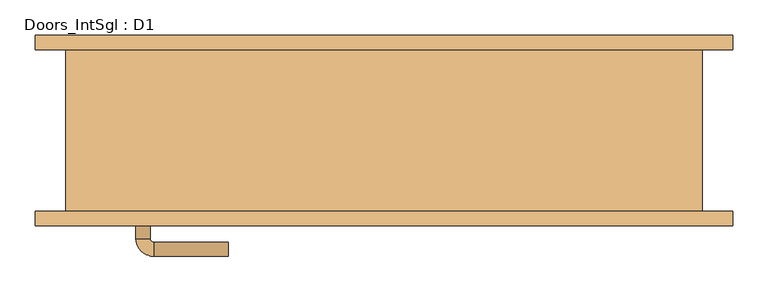
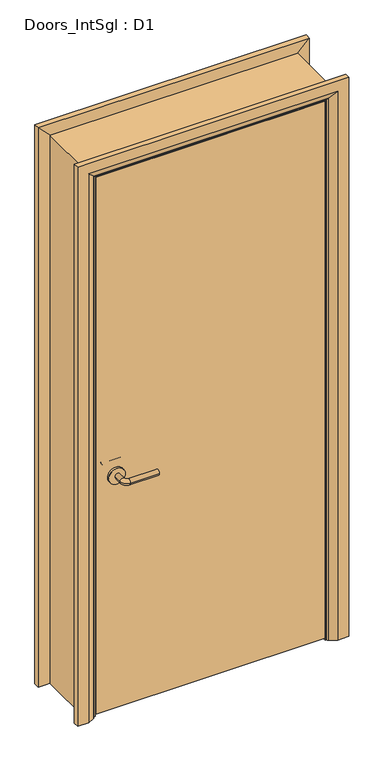
"""IFC4 building model written with IfcOpenShell, lengths in millimetres: door geometry, Doors_IntSgl : D1."""

from ifc_helpers import new_model, si_unit, point, frame, frame_2d, origin, place, context, project, spatial, polyline, circle_curve, ellipse_curve, trimmed, segment, composite_curve, outline, extrude, faceted_brep, source, transform, mapped, element, save
from ifc_brep_helpers import plane_surface, cylinder_surface, revolved_surface, advanced_brep


def doors_intsgl_d1_5aeab8eb(model_context):
    return source(origin(), model_context, "Body", "SolidModel", [
        advanced_brep(
        [(-350.2, -68.3, 900.0), (-330.2, -68.3, 900.0), (-350.2, -38.3, 900.0), (-330.2, -38.3, 900.0), (-325.2, -33.3, 900.0), (-325.2, -13.3, 900.0), (-220.2, -13.3, 900.0), (-220.2, -33.3, 900.0)],
        [
            (0, 1, circle_curve(frame((-340.2, -68.3, 900.0), z_axis=(0.0, -1.0, 0.0), x_axis=(1.0, 0.0, 0.0)), 10.0)),
            (1, 0, circle_curve(frame((-340.2, -68.3, 900.0), z_axis=(0.0, -1.0, 0.0), x_axis=(1.0, 0.0, 0.0)), 10.0)),
            (0, 2),
            (2, 3, circle_curve(frame((-340.2, -38.3, 900.0), z_axis=(0.0, -1.0, 0.0), x_axis=(1.0, 0.0, 0.0)), 10.0)),
            (3, 1),
            (3, 2, circle_curve(frame((-340.2, -38.3, 900.0), z_axis=(0.0, -1.0, 0.0), x_axis=(1.0, 0.0, 0.0)), 10.0)),
            (4, 3, circle_curve(frame((-325.2, -38.3, 900.0), z_axis=(0.0, 0.0, 1.0), x_axis=(-1.0, 0.0, 0.0)), 5.0)),
            (2, 5, circle_curve(frame((-325.2, -38.3, 900.0), z_axis=(0.0, 0.0, -1.0), x_axis=(-1.0, 0.0, 0.0)), 25.0)),
            (5, 4, circle_curve(frame((-325.2, -23.3, 900.0), z_axis=(-1.0, 0.0, 0.0), x_axis=(0.0, -1.0, 0.0)), 10.0)),
            (4, 5, circle_curve(frame((-325.2, -23.3, 900.0), z_axis=(-1.0, 0.0, 0.0), x_axis=(0.0, -1.0, 0.0)), 10.0)),
            (6, 7, circle_curve(frame((-220.2, -23.3, 900.0), z_axis=(1.0, 0.0, 0.0), x_axis=(0.0, -1.0, 0.0)), 10.0)),
            (7, 6, circle_curve(frame((-220.2, -23.3, 900.0), z_axis=(1.0, 0.0, 0.0), x_axis=(0.0, -1.0, 0.0)), 10.0)),
            (5, 6),
            (7, 4),
        ],
        [
            plane_surface(frame((-340.2, -68.3, 900.0), z_axis=(0.0, -1.0, 0.0), x_axis=(0.0, 0.0, 1.0))),
            cylinder_surface(frame((-340.2, -68.3, 900.0), z_axis=(0.0, -1.0, 0.0), x_axis=(1.0, 0.0, 0.0)), 10.0),
            revolved_surface(trimmed(ellipse_curve(frame((-340.2, -38.3, 900.0), z_axis=(0.0, -1.0, 0.0), x_axis=(1.0, 0.0, 0.0)), 10.0, 10.0), [point((-350.2, -38.3, 900.0))], [point((-330.2, -38.3, 900.0))], True, "CARTESIAN"), (-325.2, -38.3, 900.0), (0.0, 0.0, -1.0)),
            revolved_surface(trimmed(ellipse_curve(frame((-340.2, -38.3, 900.0), z_axis=(0.0, -1.0, 0.0), x_axis=(1.0, 0.0, 0.0)), 10.0, 10.0), [point((-330.2, -38.3, 900.0))], [point((-350.2, -38.3, 900.0))], True, "CARTESIAN"), (-325.2, -38.3, 900.0), (0.0, 0.0, -1.0)),
            plane_surface(frame((-220.2, -23.3, 900.0), z_axis=(1.0, 0.0, 0.0), x_axis=(0.0, 0.0, 1.0))),
            cylinder_surface(frame((-325.2, -23.3, 900.0), z_axis=(-1.0, 0.0, 0.0), x_axis=(0.0, -1.0, 0.0)), 10.0),
        ],
        [
            (0, [[1, 2]]),
            (1, [[-1, 3, 4, 5]]),
            (1, [[-2, -5, 6, -3]]),
            (2, [[7, -4, 8, 9]]),
            (3, [[-8, -6, -7, 10]]),
            (4, [[11, 12]]),
            (5, [[-9, 13, -12, 14]]),
            (5, [[-10, -14, -11, -13]]),
        ],
    ),
        extrude(outline(composite_curve([segment(trimmed(circle_curve(frame_2d((900.0, -342.7)), 30.0), [point((900.0, -372.7))], [point((900.0, -312.7))], False, "CARTESIAN"), True, "CONTINUOUS"), segment(trimmed(circle_curve(frame_2d((900.0, -342.7)), 30.0), [point((900.0, -312.7))], [point((900.0, -372.7))], False, "CARTESIAN"), True, "CONTINUOUS")], self_intersect=False)), frame((0.0, -76.3, 0.0), z_axis=(0.0, 1.0, 0.0), x_axis=(0.0, 0.0, 1.0)), (0.0, 0.0, 1.0), 8.0),
        advanced_brep(
        [(-350.2, -122.3, 900.0), (-330.2, -122.3, 900.0), (-330.2, -152.3, 900.0), (-350.2, -152.3, 900.0), (-325.2, -157.3, 900.0), (-325.2, -177.3, 900.0), (-220.2, -177.3, 900.0), (-220.2, -157.3, 900.0)],
        [
            (0, 1, circle_curve(frame((-340.2, -122.3, 900.0), z_axis=(0.0, 1.0, 0.0), x_axis=(1.0, 0.0, 0.0)), 10.0)),
            (1, 0, circle_curve(frame((-340.2, -122.3, 900.0), z_axis=(0.0, 1.0, 0.0), x_axis=(1.0, 0.0, 0.0)), 10.0)),
            (1, 2),
            (2, 3, circle_curve(frame((-340.2, -152.3, 900.0), z_axis=(0.0, 1.0, 0.0), x_axis=(1.0, 0.0, 0.0)), 10.0)),
            (3, 0),
            (3, 2, circle_curve(frame((-340.2, -152.3, 900.0), z_axis=(0.0, 1.0, 0.0), x_axis=(1.0, 0.0, 0.0)), 10.0)),
            (4, 5, circle_curve(frame((-325.2, -167.3, 900.0), z_axis=(-1.0, 0.0, 0.0), x_axis=(0.0, 1.0, 0.0)), 10.0)),
            (5, 3, circle_curve(frame((-325.2, -152.3, 900.0), z_axis=(0.0, 0.0, -1.0), x_axis=(-1.0, 0.0, 0.0)), 25.0)),
            (2, 4, circle_curve(frame((-325.2, -152.3, 900.0), z_axis=(0.0, 0.0, 1.0), x_axis=(-1.0, 0.0, 0.0)), 5.0)),
            (5, 4, circle_curve(frame((-325.2, -167.3, 900.0), z_axis=(-1.0, 0.0, 0.0), x_axis=(0.0, 1.0, 0.0)), 10.0)),
            (6, 7, circle_curve(frame((-220.2, -167.3, 900.0), z_axis=(1.0, 0.0, 0.0), x_axis=(0.0, 1.0, 0.0)), 10.0)),
            (7, 6, circle_curve(frame((-220.2, -167.3, 900.0), z_axis=(1.0, 0.0, 0.0), x_axis=(0.0, 1.0, 0.0)), 10.0)),
            (4, 7),
            (6, 5),
        ],
        [
            plane_surface(frame((-340.2, -122.3, 900.0), z_axis=(0.0, 1.0, 0.0), x_axis=(0.0, 0.0, 1.0))),
            cylinder_surface(frame((-340.2, -122.3, 900.0), z_axis=(0.0, 1.0, 0.0), x_axis=(1.0, 0.0, 0.0)), 10.0),
            revolved_surface(trimmed(ellipse_curve(frame((-340.2, -152.3, 900.0), z_axis=(0.0, -1.0, 0.0), x_axis=(1.0, 0.0, 0.0)), 10.0, 10.0), [point((-350.2, -152.3, 900.0))], [point((-330.2, -152.3, 900.0))], True, "CARTESIAN"), (-325.2, -152.3, 900.0), (0.0, 0.0, -1.0)),
            revolved_surface(trimmed(ellipse_curve(frame((-340.2, -152.3, 900.0), z_axis=(0.0, -1.0, 0.0), x_axis=(1.0, 0.0, 0.0)), 10.0, 10.0), [point((-330.2, -152.3, 900.0))], [point((-350.2, -152.3, 900.0))], True, "CARTESIAN"), (-325.2, -152.3, 900.0), (0.0, 0.0, -1.0)),
            plane_surface(frame((-220.2, -167.3, 900.0), z_axis=(1.0, 0.0, 0.0), x_axis=(0.0, 0.0, 1.0))),
            cylinder_surface(frame((-325.2, -167.3, 900.0), z_axis=(-1.0, 0.0, 0.0), x_axis=(0.0, 1.0, 0.0)), 10.0),
        ],
        [
            (0, [[1, 2]]),
            (1, [[3, 4, 5, -2]]),
            (1, [[-5, 6, -3, -1]]),
            (2, [[7, 8, -4, 9]]),
            (3, [[10, -9, -6, -8]]),
            (4, [[11, 12]]),
            (5, [[13, -11, 14, -7]]),
            (5, [[-14, -12, -13, -10]]),
        ],
    ),
        extrude(outline(composite_curve([segment(trimmed(circle_curve(frame_2d((900.0, -342.7)), 30.0), [point((900.0, -372.7))], [point((900.0, -312.7))], False, "CARTESIAN"), True, "CONTINUOUS"), segment(trimmed(circle_curve(frame_2d((900.0, -342.7)), 30.0), [point((900.0, -312.7))], [point((900.0, -372.7))], False, "CARTESIAN"), True, "CONTINUOUS")], self_intersect=False)), frame((0.0, -122.3, 0.0), z_axis=(0.0, 1.0, 0.0), x_axis=(0.0, 0.0, 1.0)), (0.0, 0.0, 1.0), 8.0),
        extrude(outline(polyline([(415.2, -76.3), (415.2, -114.3), (-415.2, -114.3), (-415.2, -76.3), (415.2, -76.3)])), frame((0.0, 0.0, 8.0), z_axis=(0.0, 0.0, 1.0), x_axis=(1.0, 0.0, 0.0)), (0.0, 0.0, 1.0), 2060.0),
        advanced_brep(
        [(492.2, -134.3, 0.0), (452.2, -134.3, 0.0), (426.2, -120.3, 0.0), (422.2, -114.3, 0.0), (492.2, -114.3, 0.0), (492.2, -114.3, 2145.0), (492.2, -134.3, 2145.0), (422.2, -114.3, 2075.0), (-422.2, -114.3, 2075.0), (-422.2, -114.3, 0.0), (-492.2, -114.3, 0.0), (-492.2, -114.3, 2145.0), (426.2, -120.3, 2079.0), (452.2, -134.3, 2105.0), (-492.2, -134.3, 2145.0), (-492.2, -134.3, 0.0), (-452.2, -134.3, 0.0), (-452.2, -134.3, 2105.0), (-426.2, -120.3, 0.0), (-426.2, -120.3, 2079.0)],
        [
            (0, 1),
            (1, 2),
            (2, 3, circle_curve(frame((430.2, -113.3, 0.0), z_axis=(0.0, 0.0, -1.0), x_axis=(1.0, 0.0, 0.0)), 8.0622577)),
            (3, 4),
            (4, 0),
            (4, 5),
            (5, 6),
            (6, 0),
            (3, 7),
            (7, 8),
            (8, 9),
            (9, 10),
            (10, 11),
            (11, 5),
            (2, 12),
            (12, 7, ellipse_curve(frame((430.2, -113.3, 2083.0), z_axis=(0.7071067811865475, 0.0, -0.7071067811865475), x_axis=(-0.7071067811865474, 0.0, -0.7071067811865476)), 11.4017543, 8.0622577)),
            (1, 13),
            (13, 12),
            (6, 14),
            (14, 15),
            (15, 16),
            (16, 17),
            (17, 13),
            (10, 15),
            (14, 11),
            (9, 18, circle_curve(frame((-430.2, -113.3, 0.0), z_axis=(0.0, 0.0, -1.0), x_axis=(-1.0, 0.0, 0.0)), 8.0622577)),
            (18, 16),
            (19, 18),
            (8, 19, ellipse_curve(frame((-430.2, -113.3, 2083.0), z_axis=(-0.7071067811865475, 0.0, -0.7071067811865475), x_axis=(-0.7071067811865474, 0.0, 0.7071067811865476)), 11.4017543, 8.0622577)),
            (19, 17),
            (12, 19),
        ],
        [
            plane_surface(frame((422.2, -114.3, 0.0), z_axis=(0.0, 0.0, -1.0), x_axis=(0.0, 1.0, 0.0))),
            plane_surface(frame((492.2, -134.3, 0.0), z_axis=(1.0, 0.0, 0.0), x_axis=(0.0, 0.0, 1.0))),
            plane_surface(frame((492.2, -114.3, 0.0), z_axis=(0.0, 1.0, 0.0), x_axis=(0.0, 0.0, 1.0))),
            cylinder_surface(frame((430.2, -113.3, 0.0), z_axis=(0.0, 0.0, -1.0), x_axis=(1.0, 0.0, 0.0)), 8.0622577),
            plane_surface(frame((426.2, -120.3, 0.0), z_axis=(-0.4740998230350126, -0.880471099922178, 0.0), x_axis=(0.0, 0.0, 1.0))),
            plane_surface(frame((452.2, -134.3, 0.0), z_axis=(0.0, -1.0, 0.0), x_axis=(0.0, 0.0, 1.0))),
            plane_surface(frame((-492.2, -134.3, 2145.0), z_axis=(-1.0, 0.0, 0.0), x_axis=(0.0, 0.0, -1.0))),
            plane_surface(frame((-422.2, -114.3, 0.0), z_axis=(0.0, 0.0, -1.0), x_axis=(0.0, 1.0, 0.0))),
            cylinder_surface(frame((-430.2, -113.3, 2075.0), z_axis=(0.0, 0.0, 1.0), x_axis=(-1.0, 0.0, 0.0)), 8.0622577),
            plane_surface(frame((-426.2, -120.3, 2079.0), z_axis=(0.47409982303501824, -0.8804710999221749, 0.0), x_axis=(0.0, 0.0, -1.0))),
            plane_surface(frame((492.2, -134.3, 2145.0), z_axis=(0.0, 0.0, 1.0), x_axis=(-1.0, 0.0, 0.0))),
            cylinder_surface(frame((422.2, -113.3, 2083.0), z_axis=(1.0, 0.0, 0.0), x_axis=(0.0, 0.0, 1.0)), 8.0622577),
            plane_surface(frame((426.2, -120.3, 2079.0), z_axis=(0.0, -0.8804710999221764, -0.4740998230350154), x_axis=(-1.0, 0.0, 0.0))),
        ],
        [
            (0, [[1, 2, 3, 4, 5]]),
            (1, [[6, 7, 8, -5]]),
            (2, [[9, 10, 11, 12, 13, 14, -6, -4]]),
            (3, [[15, 16, -9, -3]]),
            (4, [[17, 18, -15, -2]]),
            (5, [[-8, 19, 20, 21, 22, 23, -17, -1]]),
            (6, [[-13, 24, -20, 25]]),
            (7, [[-24, -12, 26, 27, -21]]),
            (8, [[28, -26, -11, 29]]),
            (9, [[-22, -27, -28, 30]]),
            (10, [[-14, -25, -19, -7]]),
            (11, [[31, -29, -10, -16]]),
            (12, [[-23, -30, -31, -18]]),
        ],
    ),
        extrude(outline(polyline([(0.0, -398.2), (2051.0, -398.2), (2051.0, 398.2), (0.0, 398.2), (0.0, 417.2), (2070.0, 417.2), (2070.0, -417.2), (0.0, -417.2), (0.0, -398.2)])), frame((0.0, -74.3, 0.0), z_axis=(0.0, 1.0, 0.0), x_axis=(0.0, 0.0, 1.0)), (0.0, 0.0, 1.0), 32.0),
        advanced_brep(
        [(-492.2, 134.3, 0.0), (-452.2, 134.3, 0.0), (-426.2, 120.3, 0.0), (-422.2, 114.3, 0.0), (-492.2, 114.3, 0.0), (-492.2, 114.3, 2145.0), (-492.2, 134.3, 2145.0), (-422.2, 114.3, 2075.0), (-426.2, 120.3, 2079.0), (-452.2, 134.3, 2105.0), (492.2, 134.3, 0.0), (492.2, 114.3, 0.0), (422.2, 114.3, 0.0), (426.2, 120.3, 0.0), (452.2, 134.3, 0.0), (492.2, 134.3, 2145.0), (452.2, 134.3, 2105.0), (426.2, 120.3, 2079.0), (422.2, 114.3, 2075.0), (492.2, 114.3, 2145.0)],
        [
            (0, 1),
            (1, 2),
            (2, 3, circle_curve(frame((-430.2, 113.3, 0.0), z_axis=(0.0, 0.0, -1.0), x_axis=(-1.0, 0.0, 0.0)), 8.0622577)),
            (3, 4),
            (4, 0),
            (4, 5),
            (5, 6),
            (6, 0),
            (3, 7),
            (7, 5),
            (2, 8),
            (8, 7, ellipse_curve(frame((-430.2, 113.3, 2083.0), z_axis=(-0.7071067811865475, 0.0, -0.7071067811865475), x_axis=(0.7071067811865474, 0.0, -0.7071067811865476)), 11.4017543, 8.0622577)),
            (1, 9),
            (9, 8),
            (6, 9),
            (10, 11),
            (11, 12),
            (12, 13, circle_curve(frame((430.2, 113.3, 0.0), z_axis=(0.0, 0.0, -1.0), x_axis=(1.0, 0.0, 0.0)), 8.0622577)),
            (13, 14),
            (14, 10),
            (15, 10),
            (14, 16),
            (16, 15),
            (13, 17),
            (17, 16),
            (12, 18),
            (18, 17, ellipse_curve(frame((430.2, 113.3, 2083.0), z_axis=(0.7071067811865475, 0.0, -0.7071067811865475), x_axis=(0.7071067811865474, 0.0, 0.7071067811865476)), 11.4017543, 8.0622577)),
            (11, 19),
            (19, 18),
            (15, 19),
            (5, 19),
            (15, 6),
            (7, 18),
            (8, 17),
            (9, 16),
        ],
        [
            plane_surface(frame((-422.2, 187.1010989, 0.0), z_axis=(0.0, 0.0, -1.0), x_axis=(1.0, 0.0, 0.0))),
            plane_surface(frame((-492.2, 134.3, 0.0), z_axis=(-1.0, 0.0, 0.0), x_axis=(0.0, 0.0, 1.0))),
            plane_surface(frame((-492.2, 114.3, 0.0), z_axis=(0.0, -1.0, 0.0), x_axis=(0.0, 0.0, 1.0))),
            cylinder_surface(frame((-430.2, 113.3, 0.0), z_axis=(0.0, 0.0, -1.0), x_axis=(-1.0, 0.0, 0.0)), 8.0622577),
            plane_surface(frame((-426.2, 120.3, 0.0), z_axis=(0.4740998230350183, 0.8804710999221749, 0.0), x_axis=(0.0, 0.0, 1.0))),
            plane_surface(frame((-452.2, 134.3, 0.0), z_axis=(0.0, 1.0, 0.0), x_axis=(0.0, 0.0, 1.0))),
            plane_surface(frame((422.2, 187.1010989, 0.0), z_axis=(0.0, 0.0, -1.0), x_axis=(-1.0, 0.0, 0.0))),
            plane_surface(frame((452.2, 134.3, 2105.0), z_axis=(0.0, 1.0, 0.0), x_axis=(0.0, 0.0, -1.0))),
            plane_surface(frame((426.2, 120.3, 2079.0), z_axis=(-0.4740998230350183, 0.8804710999221749, 0.0), x_axis=(0.0, 0.0, -1.0))),
            cylinder_surface(frame((430.2, 113.3, 2075.0), z_axis=(0.0, 0.0, 1.0), x_axis=(1.0, 0.0, 0.0)), 8.0622577),
            plane_surface(frame((492.2, 114.3, 2145.0), z_axis=(0.0, -1.0, 0.0), x_axis=(0.0, 0.0, -1.0))),
            plane_surface(frame((492.2, 134.3, 2145.0), z_axis=(1.0, 0.0, 0.0), x_axis=(0.0, 0.0, -1.0))),
            plane_surface(frame((-492.2, 134.3, 2145.0), z_axis=(0.0, 0.0, 1.0), x_axis=(1.0, 0.0, 0.0))),
            plane_surface(frame((-492.2, 114.3, 2145.0), z_axis=(0.0, -1.0, 0.0), x_axis=(1.0, 0.0, 0.0))),
            cylinder_surface(frame((-422.2, 113.3, 2083.0), z_axis=(-1.0, 0.0, 0.0), x_axis=(0.0, 0.0, 1.0)), 8.0622577),
            plane_surface(frame((-426.2, 120.3, 2079.0), z_axis=(0.0, 0.8804710999221749, -0.4740998230350183), x_axis=(1.0, 0.0, 0.0))),
            plane_surface(frame((-452.2, 134.3, 2105.0), z_axis=(0.0, 1.0, 0.0), x_axis=(1.0, 0.0, 0.0))),
        ],
        [
            (0, [[1, 2, 3, 4, 5]]),
            (1, [[6, 7, 8, -5]]),
            (2, [[9, 10, -6, -4]]),
            (3, [[11, 12, -9, -3]]),
            (4, [[13, 14, -11, -2]]),
            (5, [[-8, 15, -13, -1]]),
            (6, [[16, 17, 18, 19, 20]]),
            (7, [[21, -20, 22, 23]]),
            (8, [[-22, -19, 24, 25]]),
            (9, [[-24, -18, 26, 27]]),
            (10, [[-26, -17, 28, 29]]),
            (11, [[-28, -16, -21, 30]]),
            (12, [[31, -30, 32, -7]]),
            (13, [[33, -29, -31, -10]]),
            (14, [[34, -27, -33, -12]]),
            (15, [[35, -25, -34, -14]]),
            (16, [[-32, -23, -35, -15]]),
        ],
    ),
        faceted_brep([(-417.2, -114.3, 0.0), (-449.2, -114.3, 0.0), (-449.2, 114.3, 0.0), (-417.2, 114.3, 0.0), (-417.2, 114.3, 2070.0), (-417.2, -114.3, 2070.0), (-449.2, 114.3, 2102.0), (-449.2, -114.3, 2102.0), (417.2, -114.3, 0.0), (417.2, 114.3, 0.0), (449.2, 114.3, 0.0), (449.2, -114.3, 0.0), (417.2, -114.3, 2070.0), (449.2, -114.3, 2102.0), (449.2, 114.3, 2102.0), (417.2, 114.3, 2070.0)], [[[0, 1, 2, 3]], [[3, 4, 5, 0]], [[2, 6, 4, 3]], [[1, 7, 6, 2]], [[0, 5, 7, 1]], [[8, 9, 10, 11]], [[12, 8, 11, 13]], [[13, 11, 10, 14]], [[14, 10, 9, 15]], [[15, 9, 8, 12]], [[4, 15, 12, 5]], [[6, 14, 15, 4]], [[7, 13, 14, 6]], [[5, 12, 13, 7]]]),
    ])


if __name__ == "__main__":
    model = new_model("IFC4")
    model_context = context("Model", 3, world=origin())
    ifc_project = project(units=[si_unit("LENGTHUNIT", "METRE", prefix="MILLI")], contexts=[model_context])
    site = spatial("IfcSite", under=ifc_project)
    building = spatial("IfcBuilding", under=site)
    placement = place(None, origin())
    doors_intsgl_d1_shape = doors_intsgl_d1_5aeab8eb(model_context)
    element("IfcDoor", 1, ObjectType="Doors_IntSgl : D1", at=placement, inside=building, context=model_context, shape_type="MappedRepresentation", body=[
        mapped(doors_intsgl_d1_shape, transform((0.0, 0.0, 0.0), x_axis=(1.0, 0.0, 0.0), y_axis=(0.0, 1.0, 0.0), z_axis=(0.0, 0.0, 1.0))),
    ])
    save(model, "model.ifc")

# Revit data of these elements
# Type "Doors_IntSgl : D1"
#   Type Mark = "46"
#   Type Comments = "Internal Single"
#   Operation = "SingleSwingRight"
#   Manufacturer = "Revit"
#   Keynote = "L20"
#   Description = "Internal Single Door"
#   Analytic Construction = "Metal"
#   UnderCut = 0.026247 ft
#   Tolerance = 0.006562 ft
#   Thickness = 0.124672 ft
#   Thermal Resistance (R) = 0.270117 (m²·K)/W
#   Structural Tolerance = 0.026247 ft
#   StopDepth = 0.104987 ft
#   Stop Thickness = 0.062336 ft
#   Rough Width = 3.0 ft
#   Rough Height = 6.922572 ft
#   Height to Top Lock Rail = 3.28084 ft
#   Heat Transfer Coefficient (U) = 3.7021 W/(m²·K)
#   Handle Z Distance = 2.952756 ft
#   Handle X Distance = 0.246063 ft
#   Frame Thickness = 0.104987 ft
#   Door Panel Width = 2.724409 ft
#   Door Panel Thickness = 0.124672 ft
#   Door Panel Offset = 0.0 ft
#   Height = 6.922572 ft
#   Width = 3.0 ft
#   Door Panel Height = 6.75853 ft
#   Architrave Setback = 0.016404 ft
#   Vis - Ironmongery = yes
#   Material Ironmongery = Door - Handle
#   Material Frame = Door - Frame/Mullion (1)
#   Material Door = Door - Panel
#   Material Architrave = Door - Architrave
#   Visual Light Transmittance = 0
#   Solar Heat Gain Coefficient = 0
#   Function = (empty or 0)
#   Wall Closure = (empty or 0)
# Element 1 (IfcDoor, "Doors_IntSgl : D1")
#   Materials on its faces: "Door - Architrave", "Door - Handle", "Door - Frame/Mullion (1)", "Door - Panel"
# Materials
#   "Door - Handle": colour RGB 0 0 0, transparency 0, Keynote = "P21", Cost = 0
#   "Door - Frame/Mullion (1)": class "Wood", colour RGB 212 179 113, transparency 0, Keynote = "L20", Cost = 0
#   "Door - Panel": class "Wood", colour RGB 210 159 95, transparency 0, Keynote = "L20", Cost = 0
#   "Door - Architrave": class "Wood", colour RGB 154 90 5, transparency 0, Keynote = "P20", Cost = 0
